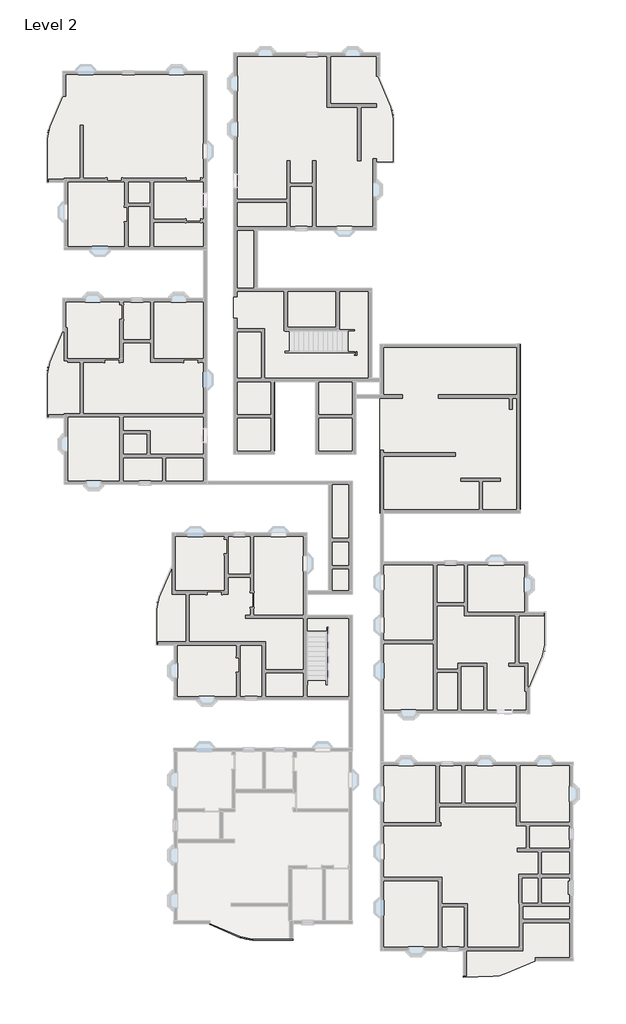
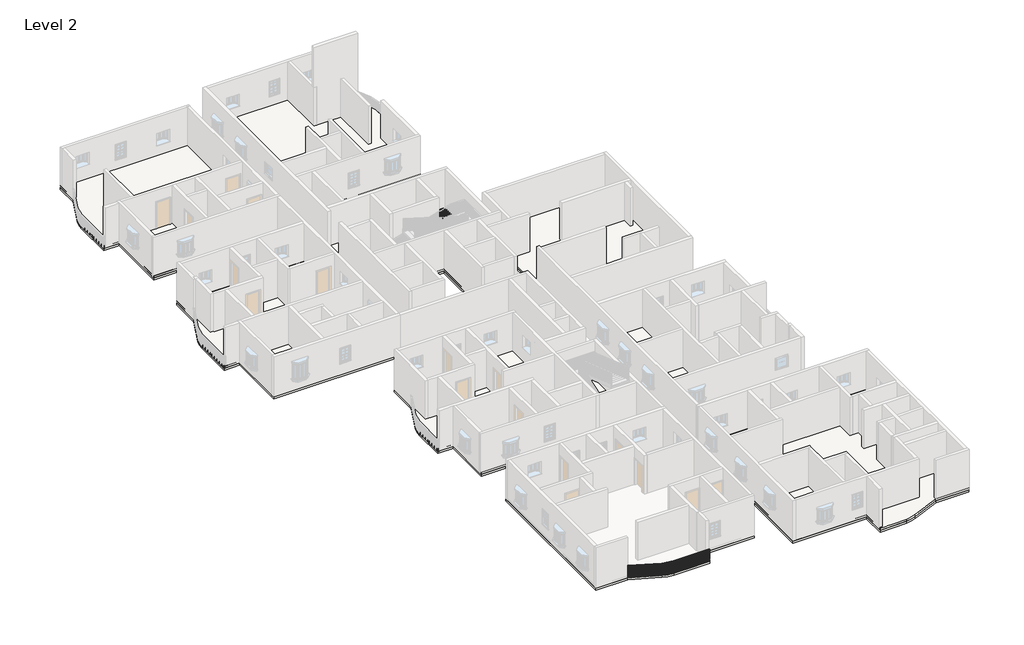
# One storey, part 5 of 14: 13 slabs, 12 roofs, 1 railing.
"""IFC4 building model written with IfcOpenShell, lengths in millimetres."""

from ifc_helpers import new_model, si_unit, point, frame, frame_2d, origin, place, context, project, spatial, polyline, circle_curve, trimmed, segment, composite_curve, outline, extrude, element, save
from ifc_brep_helpers import plane_surface, cylinder_surface, revolved_surface, advanced_brep

model = new_model("IFC4")

# Units and contexts
model_context = context("Model", 3, world=origin())
ifc_project = project(units=[si_unit("LENGTHUNIT", "METRE", prefix="MILLI")], contexts=[model_context])

# Site, building, storey
site = spatial("IfcSite", under=ifc_project)
building = spatial("IfcBuilding", under=site)
storey = spatial("IfcBuildingStorey", under=building, Name="Level 2", Elevation=3048.0)

# Railing
placement = place(None, origin())
element("IfcRailing", 1, ObjectType="Handrail - Rectangular", at=placement, inside=storey, context=model_context, shape_type="SolidModel", body=[
    advanced_brep(
    [(-10014.8722294, -25076.9923935, 3962.4), (-10014.8722294, -25076.9923935, 3911.6), (-10034.8694485, -25123.6909077, 3911.6), (-10034.8694485, -25123.6909077, 3962.4), (-8065.5370278, -25911.7359335, 3962.4), (-8065.5370278, -25911.7359335, 3911.6), (-8085.5342469, -25958.4344477, 3911.6), (-8085.5342469, -25958.4344477, 3962.4), (-7315.6413127, -26065.5416506, 3911.6), (-7315.6413127, -26065.5416506, 3962.4), (-7315.6413127, -26116.3416506, 3911.6), (-7315.6413127, -26116.3416506, 3962.4), (-4746.0891351, -26065.5416506, 3962.4), (-4746.0891351, -26116.3416506, 3962.4), (-4746.0891351, -26116.3416506, 3911.6), (-4746.0891351, -26065.5416506, 3911.6)],
    [
        (0, 1),
        (1, 2),
        (2, 3),
        (3, 0),
        (0, 4),
        (4, 5),
        (5, 1),
        (5, 6),
        (6, 2),
        (6, 7),
        (7, 3),
        (7, 4),
        (8, 5, circle_curve(frame((-7315.6413127, -24160.5416506, 3911.6), z_axis=(0.0, 0.0, -1.0), x_axis=(-0.3936460446736578, -0.9192620907623595, 0.0)), 1905.0)),
        (4, 9, circle_curve(frame((-7315.6413127, -24160.5416506, 3962.4), z_axis=(0.0, 0.0, 1.0), x_axis=(-0.3936460446736578, -0.9192620907623595, 0.0)), 1905.0)),
        (9, 8),
        (10, 6, circle_curve(frame((-7315.6413127, -24160.5416506, 3911.6), z_axis=(0.0, 0.0, -1.0), x_axis=(-0.3936460446736578, -0.9192620907623595, 0.0)), 1955.8)),
        (8, 10),
        (11, 7, circle_curve(frame((-7315.6413127, -24160.5416506, 3962.4), z_axis=(0.0, 0.0, -1.0), x_axis=(-0.3936460446736578, -0.9192620907623595, 0.0)), 1955.8)),
        (10, 11),
        (11, 9),
        (12, 13),
        (13, 14),
        (14, 15),
        (15, 12),
        (9, 12),
        (15, 8),
        (14, 10),
        (13, 11),
    ],
    [
        plane_surface(frame((-10024.8708389, -25100.3416506, 3962.4), z_axis=(-0.9192620907623597, 0.39364604467365766, 0.0), x_axis=(0.39364604467365766, 0.9192620907623597, 0.0))),
        plane_surface(frame((-10014.8722294, -25076.9923935, 3962.4), z_axis=(0.39364604467365766, 0.9192620907623597, 0.0), x_axis=(0.9192620907623597, -0.39364604467365766, 0.0))),
        plane_surface(frame((-10014.8722294, -25076.9923935, 3911.6), z_axis=(0.0, 0.0, -1.0), x_axis=(0.9192620907623597, -0.39364604467365766, 0.0))),
        plane_surface(frame((-10034.8694485, -25123.6909077, 3911.6), z_axis=(-0.39364604467365766, -0.9192620907623597, 0.0), x_axis=(0.9192620907623597, -0.39364604467365766, 0.0))),
        plane_surface(frame((-10034.8694485, -25123.6909077, 3962.4), z_axis=(0.0, 0.0, 1.0), x_axis=(0.9192620907623597, -0.39364604467365766, 0.0))),
        revolved_surface(polyline([(-8065.537027803318, -25911.735933502296, 3962.4), (-8065.537027803318, -25911.735933502296, 3911.6)]), (-7315.6413127, -24160.5416506, 3962.4), (0.0, 0.0, 1.0)),
        plane_surface(frame((-7315.6413127, -24160.5416506, 3911.6), z_axis=(0.0, 0.0, -1.0000000000000002), x_axis=(-0.3936460446736579, -0.9192620907623597, 0.0))),
        cylinder_surface(frame((-7315.6413127, -24160.5416506, 3962.4), z_axis=(0.0, 0.0, 1.0), x_axis=(-0.3936460446736578, -0.9192620907623595, 0.0)), 1955.8),
        plane_surface(frame((-7315.6413127, -24160.5416506, 3962.4), z_axis=(0.0, 0.0, 1.0000000000000002), x_axis=(-0.3936460446736579, -0.9192620907623597, 0.0))),
        plane_surface(frame((-4746.0891351, -26090.9416506, 3962.4), z_axis=(1.0, 0.0, 0.0), x_axis=(0.0, 1.0, 0.0))),
        plane_surface(frame((-7315.6413127, -26065.5416506, 3962.4), z_axis=(0.0, 1.0, 0.0), x_axis=(1.0, 0.0, 0.0))),
        plane_surface(frame((-7315.6413127, -26065.5416506, 3911.6), z_axis=(0.0, 0.0, -1.0), x_axis=(1.0, 0.0, 0.0))),
        plane_surface(frame((-7315.6413127, -26116.3416506, 3911.6), z_axis=(0.0, -1.0, 0.0), x_axis=(1.0, 0.0, 0.0))),
        plane_surface(frame((-7315.6413127, -26116.3416506, 3962.4), z_axis=(0.0, 0.0, 1.0), x_axis=(1.0, 0.0, 0.0))),
    ],
    [
        (0, [[1, 2, 3, 4]]),
        (1, [[-1, 5, 6, 7]]),
        (2, [[-2, -7, 8, 9]]),
        (3, [[-3, -9, 10, 11]]),
        (4, [[-4, -11, 12, -5]]),
        (5, [[13, -6, 14, 15]]),
        (6, [[16, -8, -13, 17]]),
        (7, [[18, -10, -16, 19]]),
        (8, [[-14, -12, -18, 20]]),
        (9, [[21, 22, 23, 24]]),
        (10, [[-15, 25, -24, 26]]),
        (11, [[-17, -26, -23, 27]]),
        (12, [[-19, -27, -22, 28]]),
        (13, [[-20, -28, -21, -25]]),
    ],
),
    extrude(outline(polyline([(-4785.1663127, -26100.4666506), (-4785.1663127, -26081.4166506), (-4766.1163127, -26081.4166506), (-4766.1163127, -26100.4666506), (-4785.1663127, -26100.4666506)])), frame((0.0, 0.0, 3048.0), z_axis=(0.0, 0.0, 1.0), x_axis=(1.0, 0.0, 0.0)), (0.0, 0.0, 1.0), 863.6),
    extrude(outline(polyline([(-4886.7663127, -26100.4666506), (-4886.7663127, -26081.4166506), (-4867.7163127, -26081.4166506), (-4867.7163127, -26100.4666506), (-4886.7663127, -26100.4666506)])), frame((0.0, 0.0, 3048.0), z_axis=(0.0, 0.0, 1.0), x_axis=(1.0, 0.0, 0.0)), (0.0, 0.0, 1.0), 863.6),
    extrude(outline(polyline([(-4988.3663127, -26100.4666506), (-4988.3663127, -26081.4166506), (-4969.3163127, -26081.4166506), (-4969.3163127, -26100.4666506), (-4988.3663127, -26100.4666506)])), frame((0.0, 0.0, 3048.0), z_axis=(0.0, 0.0, 1.0), x_axis=(1.0, 0.0, 0.0)), (0.0, 0.0, 1.0), 863.6),
    extrude(outline(polyline([(-5089.9663127, -26100.4666506), (-5089.9663127, -26081.4166506), (-5070.9163127, -26081.4166506), (-5070.9163127, -26100.4666506), (-5089.9663127, -26100.4666506)])), frame((0.0, 0.0, 3048.0), z_axis=(0.0, 0.0, 1.0), x_axis=(1.0, 0.0, 0.0)), (0.0, 0.0, 1.0), 863.6),
    extrude(outline(polyline([(-5191.5663127, -26100.4666506), (-5191.5663127, -26081.4166506), (-5172.5163127, -26081.4166506), (-5172.5163127, -26100.4666506), (-5191.5663127, -26100.4666506)])), frame((0.0, 0.0, 3048.0), z_axis=(0.0, 0.0, 1.0), x_axis=(1.0, 0.0, 0.0)), (0.0, 0.0, 1.0), 863.6),
    extrude(outline(polyline([(-5293.1663127, -26100.4666506), (-5293.1663127, -26081.4166506), (-5274.1163127, -26081.4166506), (-5274.1163127, -26100.4666506), (-5293.1663127, -26100.4666506)])), frame((0.0, 0.0, 3048.0), z_axis=(0.0, 0.0, 1.0), x_axis=(1.0, 0.0, 0.0)), (0.0, 0.0, 1.0), 863.6),
    extrude(outline(polyline([(-5394.7663127, -26100.4666506), (-5394.7663127, -26081.4166506), (-5375.7163127, -26081.4166506), (-5375.7163127, -26100.4666506), (-5394.7663127, -26100.4666506)])), frame((0.0, 0.0, 3048.0), z_axis=(0.0, 0.0, 1.0), x_axis=(1.0, 0.0, 0.0)), (0.0, 0.0, 1.0), 863.6),
    extrude(outline(polyline([(-5496.3663127, -26100.4666506), (-5496.3663127, -26081.4166506), (-5477.3163127, -26081.4166506), (-5477.3163127, -26100.4666506), (-5496.3663127, -26100.4666506)])), frame((0.0, 0.0, 3048.0), z_axis=(0.0, 0.0, 1.0), x_axis=(1.0, 0.0, 0.0)), (0.0, 0.0, 1.0), 863.6),
    extrude(outline(polyline([(-5597.9663127, -26100.4666506), (-5597.9663127, -26081.4166506), (-5578.9163127, -26081.4166506), (-5578.9163127, -26100.4666506), (-5597.9663127, -26100.4666506)])), frame((0.0, 0.0, 3048.0), z_axis=(0.0, 0.0, 1.0), x_axis=(1.0, 0.0, 0.0)), (0.0, 0.0, 1.0), 863.6),
    extrude(outline(polyline([(-5699.5663127, -26100.4666506), (-5699.5663127, -26081.4166506), (-5680.5163127, -26081.4166506), (-5680.5163127, -26100.4666506), (-5699.5663127, -26100.4666506)])), frame((0.0, 0.0, 3048.0), z_axis=(0.0, 0.0, 1.0), x_axis=(1.0, 0.0, 0.0)), (0.0, 0.0, 1.0), 863.6),
    extrude(outline(polyline([(-5801.1663127, -26100.4666506), (-5801.1663127, -26081.4166506), (-5782.1163127, -26081.4166506), (-5782.1163127, -26100.4666506), (-5801.1663127, -26100.4666506)])), frame((0.0, 0.0, 3048.0), z_axis=(0.0, 0.0, 1.0), x_axis=(1.0, 0.0, 0.0)), (0.0, 0.0, 1.0), 863.6),
    extrude(outline(polyline([(-5902.7663127, -26100.4666506), (-5902.7663127, -26081.4166506), (-5883.7163127, -26081.4166506), (-5883.7163127, -26100.4666506), (-5902.7663127, -26100.4666506)])), frame((0.0, 0.0, 3048.0), z_axis=(0.0, 0.0, 1.0), x_axis=(1.0, 0.0, 0.0)), (0.0, 0.0, 1.0), 863.6),
    extrude(outline(polyline([(-6004.3663127, -26100.4666506), (-6004.3663127, -26081.4166506), (-5985.3163127, -26081.4166506), (-5985.3163127, -26100.4666506), (-6004.3663127, -26100.4666506)])), frame((0.0, 0.0, 3048.0), z_axis=(0.0, 0.0, 1.0), x_axis=(1.0, 0.0, 0.0)), (0.0, 0.0, 1.0), 863.6),
    extrude(outline(polyline([(-6105.9663127, -26100.4666506), (-6105.9663127, -26081.4166506), (-6086.9163127, -26081.4166506), (-6086.9163127, -26100.4666506), (-6105.9663127, -26100.4666506)])), frame((0.0, 0.0, 3048.0), z_axis=(0.0, 0.0, 1.0), x_axis=(1.0, 0.0, 0.0)), (0.0, 0.0, 1.0), 863.6),
    extrude(outline(polyline([(-6207.5663127, -26100.4666506), (-6207.5663127, -26081.4166506), (-6188.5163127, -26081.4166506), (-6188.5163127, -26100.4666506), (-6207.5663127, -26100.4666506)])), frame((0.0, 0.0, 3048.0), z_axis=(0.0, 0.0, 1.0), x_axis=(1.0, 0.0, 0.0)), (0.0, 0.0, 1.0), 863.6),
    extrude(outline(polyline([(-6309.1663127, -26100.4666506), (-6309.1663127, -26081.4166506), (-6290.1163127, -26081.4166506), (-6290.1163127, -26100.4666506), (-6309.1663127, -26100.4666506)])), frame((0.0, 0.0, 3048.0), z_axis=(0.0, 0.0, 1.0), x_axis=(1.0, 0.0, 0.0)), (0.0, 0.0, 1.0), 863.6),
    extrude(outline(polyline([(-6410.7663127, -26100.4666506), (-6410.7663127, -26081.4166506), (-6391.7163127, -26081.4166506), (-6391.7163127, -26100.4666506), (-6410.7663127, -26100.4666506)])), frame((0.0, 0.0, 3048.0), z_axis=(0.0, 0.0, 1.0), x_axis=(1.0, 0.0, 0.0)), (0.0, 0.0, 1.0), 863.6),
    extrude(outline(polyline([(-6512.3663127, -26100.4666506), (-6512.3663127, -26081.4166506), (-6493.3163127, -26081.4166506), (-6493.3163127, -26100.4666506), (-6512.3663127, -26100.4666506)])), frame((0.0, 0.0, 3048.0), z_axis=(0.0, 0.0, 1.0), x_axis=(1.0, 0.0, 0.0)), (0.0, 0.0, 1.0), 863.6),
    extrude(outline(polyline([(-6613.9663127, -26100.4666506), (-6613.9663127, -26081.4166506), (-6594.9163127, -26081.4166506), (-6594.9163127, -26100.4666506), (-6613.9663127, -26100.4666506)])), frame((0.0, 0.0, 3048.0), z_axis=(0.0, 0.0, 1.0), x_axis=(1.0, 0.0, 0.0)), (0.0, 0.0, 1.0), 863.6),
    extrude(outline(polyline([(-6715.5663127, -26100.4666506), (-6715.5663127, -26081.4166506), (-6696.5163127, -26081.4166506), (-6696.5163127, -26100.4666506), (-6715.5663127, -26100.4666506)])), frame((0.0, 0.0, 3048.0), z_axis=(0.0, 0.0, 1.0), x_axis=(1.0, 0.0, 0.0)), (0.0, 0.0, 1.0), 863.6),
    extrude(outline(polyline([(-6817.1663127, -26100.4666506), (-6817.1663127, -26081.4166506), (-6798.1163127, -26081.4166506), (-6798.1163127, -26100.4666506), (-6817.1663127, -26100.4666506)])), frame((0.0, 0.0, 3048.0), z_axis=(0.0, 0.0, 1.0), x_axis=(1.0, 0.0, 0.0)), (0.0, 0.0, 1.0), 863.6),
    extrude(outline(polyline([(-6918.7663127, -26100.4666506), (-6918.7663127, -26081.4166506), (-6899.7163127, -26081.4166506), (-6899.7163127, -26100.4666506), (-6918.7663127, -26100.4666506)])), frame((0.0, 0.0, 3048.0), z_axis=(0.0, 0.0, 1.0), x_axis=(1.0, 0.0, 0.0)), (0.0, 0.0, 1.0), 863.6),
    extrude(outline(polyline([(-7020.3663127, -26100.4666506), (-7020.3663127, -26081.4166506), (-7001.3163127, -26081.4166506), (-7001.3163127, -26100.4666506), (-7020.3663127, -26100.4666506)])), frame((0.0, 0.0, 3048.0), z_axis=(0.0, 0.0, 1.0), x_axis=(1.0, 0.0, 0.0)), (0.0, 0.0, 1.0), 863.6),
    extrude(outline(polyline([(-7121.9663127, -26100.4666506), (-7121.9663127, -26081.4166506), (-7102.9163127, -26081.4166506), (-7102.9163127, -26100.4666506), (-7121.9663127, -26100.4666506)])), frame((0.0, 0.0, 3048.0), z_axis=(0.0, 0.0, 1.0), x_axis=(1.0, 0.0, 0.0)), (0.0, 0.0, 1.0), 863.6),
    extrude(outline(polyline([(-7223.5663127, -26100.4666506), (-7223.5663127, -26081.4166506), (-7204.5163127, -26081.4166506), (-7204.5163127, -26100.4666506), (-7223.5663127, -26100.4666506)])), frame((0.0, 0.0, 3048.0), z_axis=(0.0, 0.0, 1.0), x_axis=(1.0, 0.0, 0.0)), (0.0, 0.0, 1.0), 863.6),
    extrude(outline(polyline([(-7395.3185803, -26098.8530973), (-7394.6296262, -26079.8155596), (-7375.5920885, -26080.5045137), (-7376.2810426, -26099.5420514), (-7395.3185803, -26098.8530973)])), frame((0.0, 0.0, 3048.0), z_axis=(0.0, 0.0, 1.0), x_axis=(1.0, 0.0, 0.0)), (0.0, 0.0, 1.0), 863.6),
    extrude(outline(polyline([(-7497.177549, -26091.9774704), (-7495.4880357, -26073.0025384), (-7476.5131037, -26074.6920517), (-7478.2026169, -26093.6669837), (-7497.177549, -26091.9774704)])), frame((0.0, 0.0, 3048.0), z_axis=(0.0, 0.0, 1.0), x_axis=(1.0, 0.0, 0.0)), (0.0, 0.0, 1.0), 863.6),
    extrude(outline(polyline([(-7598.5337632, -26079.7528408), (-7595.8483698, -26060.8930645), (-7576.9885935, -26063.5784579), (-7579.6739869, -26082.4382342), (-7598.5337632, -26079.7528408)])), frame((0.0, 0.0, 3048.0), z_axis=(0.0, 0.0, 1.0), x_axis=(1.0, 0.0, 0.0)), (0.0, 0.0, 1.0), 863.6),
    extrude(outline(polyline([(-7699.1065227, -26062.2130639), (-7695.4326862, -26043.5206744), (-7676.7402967, -26047.1945108), (-7680.4141332, -26065.8869003), (-7699.1065227, -26062.2130639)])), frame((0.0, 0.0, 3048.0), z_axis=(0.0, 0.0, 1.0), x_axis=(1.0, 0.0, 0.0)), (0.0, 0.0, 1.0), 863.6),
    extrude(outline(polyline([(-7798.6172969, -26039.4067149), (-7793.9651918, -26020.9334797), (-7775.4919566, -26025.5855848), (-7780.1440617, -26044.05882), (-7798.6172969, -26039.4067149)])), frame((0.0, 0.0, 3048.0), z_axis=(0.0, 0.0, 1.0), x_axis=(1.0, 0.0, 0.0)), (0.0, 0.0, 1.0), 863.6),
    extrude(outline(polyline([(-7896.7904963, -26011.396955), (-7891.1730064, -25993.1940347), (-7872.9700861, -25998.8115246), (-7878.587576, -26017.0144449), (-7896.7904963, -26011.396955)])), frame((0.0, 0.0, 3048.0), z_axis=(0.0, 0.0, 1.0), x_axis=(1.0, 0.0, 0.0)), (0.0, 0.0, 1.0), 863.6),
    extrude(outline(polyline([(-7993.3542357, -25978.2613554), (-7986.7869183, -25960.379162), (-7968.9047249, -25966.9464794), (-7975.4720423, -25984.8286729), (-7993.3542357, -25978.2613554)])), frame((0.0, 0.0, 3048.0), z_axis=(0.0, 0.0, 1.0), x_axis=(1.0, 0.0, 0.0)), (0.0, 0.0, 1.0), 863.6),
    extrude(outline(polyline([(-8169.4357205, -25905.2369062), (-8161.9367633, -25887.7249634), (-8144.4248205, -25895.2239205), (-8151.9237777, -25912.7358634), (-8169.4357205, -25905.2369062)])), frame((0.0, 0.0, 3048.0), z_axis=(0.0, 0.0, 1.0), x_axis=(1.0, 0.0, 0.0)), (0.0, 0.0, 1.0), 863.6),
    extrude(outline(polyline([(-8262.8327489, -25865.2424681), (-8255.3337918, -25847.7305252), (-8237.8218489, -25855.2294824), (-8245.3208061, -25872.7414252), (-8262.8327489, -25865.2424681)])), frame((0.0, 0.0, 3048.0), z_axis=(0.0, 0.0, 1.0), x_axis=(1.0, 0.0, 0.0)), (0.0, 0.0, 1.0), 863.6),
    extrude(outline(polyline([(-8356.2297773, -25825.2480299), (-8348.7308202, -25807.7360871), (-8331.2188774, -25815.2350443), (-8338.7178345, -25832.7469871), (-8356.2297773, -25825.2480299)])), frame((0.0, 0.0, 3048.0), z_axis=(0.0, 0.0, 1.0), x_axis=(1.0, 0.0, 0.0)), (0.0, 0.0, 1.0), 863.6),
    extrude(outline(polyline([(-8449.6268058, -25785.2535918), (-8442.1278486, -25767.741649), (-8424.6159058, -25775.2406061), (-8432.1148629, -25792.752549), (-8449.6268058, -25785.2535918)])), frame((0.0, 0.0, 3048.0), z_axis=(0.0, 0.0, 1.0), x_axis=(1.0, 0.0, 0.0)), (0.0, 0.0, 1.0), 863.6),
    extrude(outline(polyline([(-8543.0238342, -25745.2591537), (-8535.524877, -25727.7472108), (-8518.0129342, -25735.246168), (-8525.5118914, -25752.7581108), (-8543.0238342, -25745.2591537)])), frame((0.0, 0.0, 3048.0), z_axis=(0.0, 0.0, 1.0), x_axis=(1.0, 0.0, 0.0)), (0.0, 0.0, 1.0), 863.6),
    extrude(outline(polyline([(-8636.4208626, -25705.2647155), (-8628.9219055, -25687.7527727), (-8611.4099626, -25695.2517298), (-8618.9089198, -25712.7636727), (-8636.4208626, -25705.2647155)])), frame((0.0, 0.0, 3048.0), z_axis=(0.0, 0.0, 1.0), x_axis=(1.0, 0.0, 0.0)), (0.0, 0.0, 1.0), 863.6),
    extrude(outline(polyline([(-8729.817891, -25665.2702774), (-8722.3189339, -25647.7583346), (-8704.806991, -25655.2572917), (-8712.3059482, -25672.7692345), (-8729.817891, -25665.2702774)])), frame((0.0, 0.0, 3048.0), z_axis=(0.0, 0.0, 1.0), x_axis=(1.0, 0.0, 0.0)), (0.0, 0.0, 1.0), 863.6),
    extrude(outline(polyline([(-8823.2149194, -25625.2758392), (-8815.7159623, -25607.7638964), (-8798.2040195, -25615.2628536), (-8805.7029766, -25632.7747964), (-8823.2149194, -25625.2758392)])), frame((0.0, 0.0, 3048.0), z_axis=(0.0, 0.0, 1.0), x_axis=(1.0, 0.0, 0.0)), (0.0, 0.0, 1.0), 863.6),
    extrude(outline(polyline([(-8916.6119479, -25585.2814011), (-8909.1129907, -25567.7694583), (-8891.6010479, -25575.2684154), (-8899.100005, -25592.7803583), (-8916.6119479, -25585.2814011)])), frame((0.0, 0.0, 3048.0), z_axis=(0.0, 0.0, 1.0), x_axis=(1.0, 0.0, 0.0)), (0.0, 0.0, 1.0), 863.6),
    extrude(outline(polyline([(-9010.0089763, -25545.286963), (-9002.5100191, -25527.7750201), (-8984.9980763, -25535.2739773), (-8992.4970335, -25552.7859201), (-9010.0089763, -25545.286963)])), frame((0.0, 0.0, 3048.0), z_axis=(0.0, 0.0, 1.0), x_axis=(1.0, 0.0, 0.0)), (0.0, 0.0, 1.0), 863.6),
    extrude(outline(polyline([(-9103.4060047, -25505.2925248), (-9095.9070476, -25487.780582), (-9078.3951047, -25495.2795391), (-9085.8940619, -25512.791482), (-9103.4060047, -25505.2925248)])), frame((0.0, 0.0, 3048.0), z_axis=(0.0, 0.0, 1.0), x_axis=(1.0, 0.0, 0.0)), (0.0, 0.0, 1.0), 863.6),
    extrude(outline(polyline([(-9196.8030331, -25465.2980867), (-9189.304076, -25447.7861439), (-9171.7921332, -25455.285101), (-9179.2910903, -25472.7970438), (-9196.8030331, -25465.2980867)])), frame((0.0, 0.0, 3048.0), z_axis=(0.0, 0.0, 1.0), x_axis=(1.0, 0.0, 0.0)), (0.0, 0.0, 1.0), 863.6),
    extrude(outline(polyline([(-9290.2000616, -25425.3036485), (-9282.7011044, -25407.7917057), (-9265.1891616, -25415.2906629), (-9272.6881187, -25432.8026057), (-9290.2000616, -25425.3036485)])), frame((0.0, 0.0, 3048.0), z_axis=(0.0, 0.0, 1.0), x_axis=(1.0, 0.0, 0.0)), (0.0, 0.0, 1.0), 863.6),
    extrude(outline(polyline([(-9383.59709, -25385.3092104), (-9376.0981328, -25367.7972676), (-9358.58619, -25375.2962247), (-9366.0851471, -25392.8081676), (-9383.59709, -25385.3092104)])), frame((0.0, 0.0, 3048.0), z_axis=(0.0, 0.0, 1.0), x_axis=(1.0, 0.0, 0.0)), (0.0, 0.0, 1.0), 863.6),
    extrude(outline(polyline([(-9476.9941184, -25345.3147723), (-9469.4951612, -25327.8028294), (-9451.9832184, -25335.3017866), (-9459.4821756, -25352.8137294), (-9476.9941184, -25345.3147723)])), frame((0.0, 0.0, 3048.0), z_axis=(0.0, 0.0, 1.0), x_axis=(1.0, 0.0, 0.0)), (0.0, 0.0, 1.0), 863.6),
    extrude(outline(polyline([(-9570.3911468, -25305.3203341), (-9562.8921897, -25287.8083913), (-9545.3802468, -25295.3073485), (-9552.879204, -25312.8192913), (-9570.3911468, -25305.3203341)])), frame((0.0, 0.0, 3048.0), z_axis=(0.0, 0.0, 1.0), x_axis=(1.0, 0.0, 0.0)), (0.0, 0.0, 1.0), 863.6),
    extrude(outline(polyline([(-9663.7881752, -25265.325896), (-9656.2892181, -25247.8139532), (-9638.7772753, -25255.3129103), (-9646.2762324, -25272.8248531), (-9663.7881752, -25265.325896)])), frame((0.0, 0.0, 3048.0), z_axis=(0.0, 0.0, 1.0), x_axis=(1.0, 0.0, 0.0)), (0.0, 0.0, 1.0), 863.6),
    extrude(outline(polyline([(-9757.1852037, -25225.3314579), (-9749.6862465, -25207.819515), (-9732.1743037, -25215.3184722), (-9739.6732608, -25232.830415), (-9757.1852037, -25225.3314579)])), frame((0.0, 0.0, 3048.0), z_axis=(0.0, 0.0, 1.0), x_axis=(1.0, 0.0, 0.0)), (0.0, 0.0, 1.0), 863.6),
    extrude(outline(polyline([(-9850.5822321, -25185.3370197), (-9843.0832749, -25167.8250769), (-9825.5713321, -25175.324034), (-9833.0702893, -25192.8359769), (-9850.5822321, -25185.3370197)])), frame((0.0, 0.0, 3048.0), z_axis=(0.0, 0.0, 1.0), x_axis=(1.0, 0.0, 0.0)), (0.0, 0.0, 1.0), 863.6),
    extrude(outline(polyline([(-9943.9792605, -25145.3425816), (-9936.4803034, -25127.8306387), (-9918.9683605, -25135.3295959), (-9926.4673177, -25152.8415387), (-9943.9792605, -25145.3425816)])), frame((0.0, 0.0, 3048.0), z_axis=(0.0, 0.0, 1.0), x_axis=(1.0, 0.0, 0.0)), (0.0, 0.0, 1.0), 863.6),
    extrude(outline(polyline([(-7325.1663127, -26100.4666506), (-7325.1663127, -26081.4166506), (-7306.1163127, -26081.4166506), (-7306.1163127, -26100.4666506), (-7325.1663127, -26100.4666506)])), frame((0.0, 0.0, 3048.0), z_axis=(0.0, 0.0, 1.0), x_axis=(1.0, 0.0, 0.0)), (0.0, 0.0, 1.0), 863.6),
    extrude(outline(polyline([(-8088.0410874, -25940.0916834), (-8080.5421302, -25922.5797406), (-8063.0301874, -25930.0786978), (-8070.5291445, -25947.5906406), (-8088.0410874, -25940.0916834)])), frame((0.0, 0.0, 3048.0), z_axis=(0.0, 0.0, 1.0), x_axis=(1.0, 0.0, 0.0)), (0.0, 0.0, 1.0), 863.6),
    extrude(outline(polyline([(-4765.1391351, -26100.4666506), (-4765.1391351, -26081.4166506), (-4746.0891351, -26081.4166506), (-4746.0891351, -26100.4666506), (-4765.1391351, -26100.4666506)])), frame((0.0, 0.0, 3048.0), z_axis=(0.0, 0.0, 1.0), x_axis=(1.0, 0.0, 0.0)), (0.0, 0.0, 1.0), 863.6),
    extrude(outline(polyline([(-10028.6203175, -25109.097622), (-10021.1213604, -25091.5856792), (-10003.6094175, -25099.0846363), (-10011.1083747, -25116.5965792), (-10028.6203175, -25109.097622)])), frame((0.0, 0.0, 3048.0), z_axis=(0.0, 0.0, 1.0), x_axis=(1.0, 0.0, 0.0)), (0.0, 0.0, 1.0), 863.6),
])

# Roofs
element("IfcRoof", 2, ObjectType="Generic - 12\"", at=placement, inside=storey, context=model_context, shape_type="SweptSolid", body=[
    extrude(outline(composite_curve([segment(polyline([(6070.4380523, -26783.9042694), (812.6380523, -26783.9042694), (812.6380523, -14845.9042694), (13017.3380523, -14845.9042694), (13017.3380523, -27431.6042694), (10660.5280667, -27431.6042694), (8711.1928652, -28266.3478094)]), True, "CONTINUOUS"), segment(trimmed(circle_curve(frame_2d((7951.2985405, -26491.8042694)), 1930.4), [point((8711.1928652, -28266.3478094))], [point((7953.0959373, -28422.2034326))], False, "CARTESIAN"), True, "CONTINUOUS"), segment(polyline([(7953.0959373, -28422.2034326), (6070.4380523, -28487.9472947), (6070.4380523, -26783.9042694)]), True, "CONTINUOUS")], self_intersect=False)), frame((0.0, 0.0, 3048.0), z_axis=(0.0, 0.0, 1.0), x_axis=(1.0, 0.0, 0.0)), (0.0, 0.0, 1.0), 152.4),
])
element("IfcRoof", 3, ObjectType="Generic - 12\"", at=placement, inside=storey, context=model_context, shape_type="SweptSolid", body=[
    extrude(outline(composite_curve([segment(polyline([(10274.1380523, -11759.8042694), (803.8108649, -11759.8042694), (803.8108649, -2133.2042694), (10159.8380523, -2133.2042694), (10159.8380523, -5352.6542694), (11264.7380523, -5352.6542694), (11264.7380523, -7397.5810633)]), True, "CONTINUOUS"), segment(trimmed(circle_curve(frame_2d((9334.3380523, -7397.5810633)), 1930.4), [point((11264.7380523, -7397.5810633))], [point((11108.8815923, -8157.475388))], False, "CARTESIAN"), True, "CONTINUOUS"), segment(polyline([(11108.8815923, -8157.475388), (10274.1380523, -10106.8105895), (10274.1380523, -11759.8042694)]), True, "CONTINUOUS")], self_intersect=False)), frame((0.0, 0.0, 3048.0), z_axis=(0.0, 0.0, 1.0), x_axis=(1.0, 0.0, 0.0)), (0.0, 0.0, 1.0), 152.4),
])
element("IfcRoof", 4, ObjectType="Generic - 12\"", at=placement, inside=storey, context=model_context, shape_type="SweptSolid", body=[
    extrude(outline(composite_curve([segment(polyline([(-13395.387215, -7421.9416506), (-13395.387215, -5140.4900045)]), True, "CONTINUOUS"), segment(trimmed(circle_curve(frame_2d((-11464.987215, -5140.4900045)), 1930.4), [point((-13395.387215, -5140.4900045))], [point((-13239.530755, -4380.5956799))], False, "CARTESIAN"), True, "CONTINUOUS"), segment(polyline([(-13239.530755, -4380.5956799), (-12404.787215, -2431.2604783), (-12404.787215, -322.6416506), (-3857.687215, -322.6416506), (-3857.687215, -5523.2916506), (-974.1891351, -5523.2916506), (-974.1891351, -10889.0416506), (-12290.487215, -10889.0416506), (-12290.487215, -7421.9416506), (-13395.387215, -7421.9416506)]), True, "CONTINUOUS")], self_intersect=False)), frame((0.0, 0.0, 3048.0), z_axis=(0.0, 0.0, 1.0), x_axis=(1.0, 0.0, 0.0)), (0.0, 0.0, 1.0), 152.4),
])
element("IfcRoof", 5, ObjectType="Generic - 12\"", at=placement, inside=storey, context=model_context, shape_type="SweptSolid", body=[
    extrude(outline(polyline([(-2472.7891351, 2953.9583494), (-961.4891351, 2953.9583494), (-961.4891351, -4202.4916506), (-2472.7891351, -4202.4916506), (-2472.7891351, 2953.9583494)])), frame((0.0, 0.0, 3048.0), z_axis=(0.0, 0.0, 1.0), x_axis=(1.0, 0.0, 0.0)), (0.0, 0.0, 1.0), 152.4),
])
element("IfcRoof", 6, ObjectType="Generic - 12\"", at=placement, inside=storey, context=model_context, shape_type="SweptSolid", body=[
    extrude(outline(composite_curve([segment(polyline([(-10194.3891351, 2750.7583494), (-19236.7891351, 2750.7583494), (-19236.7891351, 6979.8583494), (-20341.6891351, 6979.8583494), (-20341.6891351, 9746.7948172)]), True, "CONTINUOUS"), segment(trimmed(circle_curve(frame_2d((-18411.2891351, 9746.7948172)), 1930.4), [point((-20341.6891351, 9746.7948172))], [point((-20185.8326751, 10506.6891419))], False, "CARTESIAN"), True, "CONTINUOUS"), segment(polyline([(-20185.8326751, 10506.6891419), (-19351.0891351, 12456.0243434), (-19351.0891351, 14536.3583494), (-10194.3891351, 14536.3583494), (-10194.3891351, 2750.7583494)]), True, "CONTINUOUS")], self_intersect=False)), frame((0.0, 0.0, 3048.0), z_axis=(0.0, 0.0, 1.0), x_axis=(1.0, 0.0, 0.0)), (0.0, 0.0, 1.0), 152.4),
])
element("IfcRoof", 7, ObjectType="Generic - 12\"", at=placement, inside=storey, context=model_context, shape_type="SweptSolid", body=[
    extrude(outline(composite_curve([segment(polyline([(-10194.3891351, 17609.7583494), (-19236.7891351, 17609.7583494), (-19236.7891351, 21889.6583494), (-20341.6891351, 21889.6583494), (-20341.6891351, 24656.5948172)]), True, "CONTINUOUS"), segment(trimmed(circle_curve(frame_2d((-18411.2891351, 24656.5948172)), 1930.4), [point((-20341.6891351, 24656.5948172))], [point((-20185.8326751, 25416.4891419))], False, "CARTESIAN"), True, "CONTINUOUS"), segment(polyline([(-20185.8326751, 25416.4891419), (-19351.0891351, 27365.8243434), (-19351.0891351, 28950.8583494), (-10194.3891351, 28950.8583494), (-10194.3891351, 17609.7583494)]), True, "CONTINUOUS")], self_intersect=False)), frame((0.0, 0.0, 3048.0), z_axis=(0.0, 0.0, 1.0), x_axis=(1.0, 0.0, 0.0)), (0.0, 0.0, 1.0), 152.4),
])
element("IfcRoof", 8, ObjectType="Generic - 12\"", at=placement, inside=storey, context=model_context, shape_type="SweptSolid", body=[
    extrude(outline(composite_curve([segment(polyline([(-8492.5891351, 18875.1215905), (-8492.5891351, 30101.9215905), (664.1108649, 30101.9215905), (664.1108649, 28631.1875845), (1498.8544049, 26681.8523829)]), True, "CONTINUOUS"), segment(trimmed(circle_curve(frame_2d((-275.6891351, 25921.9580583)), 1930.4), [point((1498.8544049, 26681.8523829))], [point((1654.7108649, 25921.9580583))], False, "CARTESIAN"), True, "CONTINUOUS"), segment(polyline([(1654.7108649, 25921.9580583), (1654.7108649, 23155.0215905), (549.8108649, 23155.0215905), (549.8108649, 18875.1215905), (-8492.5891351, 18875.1215905)]), True, "CONTINUOUS")], self_intersect=False)), frame((0.0, 0.0, 3048.0), z_axis=(0.0, 0.0, 1.0), x_axis=(1.0, 0.0, 0.0)), (0.0, 0.0, 1.0), 152.4),
])
element("IfcRoof", 9, ObjectType="Generic - 12\"", at=placement, inside=storey, context=model_context, shape_type="SweptSolid", body=[
    extrude(outline(polyline([(-8492.5891351, 9478.4949943), (-5914.4891351, 9478.4949943), (-5914.4891351, 4665.1949943), (-8492.5891351, 4665.1949943), (-8492.5891351, 9478.4949943)])), frame((0.0, 0.0, 3048.0), z_axis=(0.0, 0.0, 1.0), x_axis=(1.0, 0.0, 0.0)), (0.0, 0.0, 1.0), 152.4),
])
element("IfcRoof", 10, ObjectType="Generic - 12\"", at=placement, inside=storey, context=model_context, shape_type="SweptSolid", body=[
    extrude(outline(polyline([(-3310.9891351, 9478.4949943), (-745.5891351, 9478.4949943), (-745.5891351, 4652.4949943), (-3310.9891351, 4652.4949943), (-3310.9891351, 9478.4949943)])), frame((0.0, 0.0, 3048.0), z_axis=(0.0, 0.0, 1.0), x_axis=(1.0, 0.0, 0.0)), (0.0, 0.0, 1.0), 152.4),
])
element("IfcRoof", 11, ObjectType="Generic - 12\"", at=placement, inside=storey, context=model_context, shape_type="SweptSolid", body=[
    extrude(outline(polyline([(-8492.5891351, 19078.3215905), (-6993.9891351, 19078.3215905), (-6993.9891351, 14988.9215905), (-8492.5891351, 14988.9215905), (-8492.5891351, 19078.3215905)])), frame((0.0, 0.0, 3048.0), z_axis=(0.0, 0.0, 1.0), x_axis=(1.0, 0.0, 0.0)), (0.0, 0.0, 1.0), 152.4),
])
element("IfcRoof", 12, ObjectType="Generic - 12\"", at=placement, inside=storey, context=model_context, shape_type="SweptSolid", body=[
    extrude(outline(polyline([(-8492.5891351, 15192.1215905), (257.7108649, 15192.1215905), (257.7108649, 9275.2949943), (-8492.5891351, 9275.2949943), (-8492.5891351, 15192.1215905)])), frame((0.0, 0.0, 3048.0), z_axis=(0.0, 0.0, 1.0), x_axis=(1.0, 0.0, 0.0)), (0.0, 0.0, 1.0), 152.4),
])
element("IfcRoof", 13, ObjectType="Generic - 12\"", at=placement, inside=storey, context=model_context, shape_type="SweptSolid", body=[
    extrude(outline(polyline([(793.5880523, 11646.2957306), (9677.2380523, 11646.2957306), (9677.2380523, 940.1957306), (793.5880523, 940.1957306), (793.5880523, 11646.2957306)])), frame((0.0, 0.0, 3048.0), z_axis=(0.0, 0.0, 1.0), x_axis=(1.0, 0.0, 0.0)), (0.0, 0.0, 1.0), 152.4),
])

# Slabs
element("IfcSlab", 14, ObjectType="Generic - 12\"", at=placement, inside=storey, context=model_context, shape_type="SweptSolid", body=[
    extrude(outline(composite_curve([segment(polyline([(-20341.6891351, 21889.6583494), (-20341.6891351, 24656.5948172)]), True, "CONTINUOUS"), segment(trimmed(circle_curve(frame_2d((-18411.2891351, 24656.5948172)), 1930.4), [point((-20341.6891351, 24656.5948172))], [point((-20185.8326751, 25416.4891419))], False, "CARTESIAN"), True, "CONTINUOUS"), segment(polyline([(-20185.8326751, 25416.4891419), (-19351.0891351, 27365.8243434), (-19351.0891351, 28950.8583494), (-10194.3891351, 28950.8583494), (-10194.3891351, 17609.7583494), (-19236.7891351, 17609.7583494), (-19236.7891351, 21889.6583494), (-20341.6891351, 21889.6583494)]), True, "CONTINUOUS")], self_intersect=False)), frame((0.0, 0.0, 2895.6), z_axis=(0.0, 0.0, 1.0), x_axis=(1.0, 0.0, 0.0)), (0.0, 0.0, 1.0), 152.4),
])
element("IfcSlab", 15, ObjectType="Generic - 12\"", at=placement, inside=storey, context=model_context, shape_type="SweptSolid", body=[
    extrude(outline(composite_curve([segment(polyline([(-10024.8708389, -25100.3416506), (-12290.487215, -25100.3416506), (-12290.487215, -13962.4416506), (-986.8891351, -13962.4416506), (-986.8891351, -25100.3416506), (-4746.0891351, -25100.3416506), (-4746.0891351, -26090.9416506), (-7315.6413127, -26090.9416506)]), True, "CONTINUOUS"), segment(trimmed(circle_curve(frame_2d((-7315.6413127, -24160.5416506)), 1930.4), [point((-7315.6413127, -26090.9416506))], [point((-8075.5356374, -25935.0851906))], False, "CARTESIAN"), True, "CONTINUOUS"), segment(polyline([(-8075.5356374, -25935.0851906), (-10024.8708389, -25100.3416506)]), True, "CONTINUOUS")], self_intersect=False)), frame((0.0, 0.0, 2895.6), z_axis=(0.0, 0.0, 1.0), x_axis=(1.0, 0.0, 0.0)), (0.0, 0.0, 1.0), 152.4),
])
element("IfcSlab", 16, ObjectType="Generic - 12\"", at=placement, inside=storey, context=model_context, shape_type="SweptSolid", body=[
    extrude(outline(composite_curve([segment(polyline([(13017.3380523, -27431.6042694), (10660.5280667, -27431.6042694), (8711.1928652, -28266.3478094)]), True, "CONTINUOUS"), segment(trimmed(circle_curve(frame_2d((7951.2985405, -26491.8042694)), 1930.4), [point((8711.1928652, -28266.3478094))], [point((7953.0959373, -28422.2034326))], False, "CARTESIAN"), True, "CONTINUOUS"), segment(polyline([(7953.0959373, -28422.2034326), (6070.4380523, -28487.9472947), (6070.4380523, -26783.9042694), (812.6380523, -26783.9042694), (812.6380523, -14845.9042694), (13017.3380523, -14845.9042694), (13017.3380523, -27431.6042694)]), True, "CONTINUOUS")], self_intersect=False)), frame((0.0, 0.0, 2895.6), z_axis=(0.0, 0.0, 1.0), x_axis=(1.0, 0.0, 0.0)), (0.0, 0.0, 1.0), 152.4),
])
element("IfcSlab", 17, ObjectType="Generic - 12\"", at=placement, inside=storey, context=model_context, shape_type="SweptSolid", body=[
    extrude(outline(composite_curve([segment(polyline([(10274.1380523, -11759.8042694), (803.8108649, -11759.8042694), (803.8108649, -2133.2042694), (10159.8380523, -2133.2042694), (10159.8380523, -5352.6542694), (11264.7380523, -5352.6542694), (11264.7380523, -7397.5810633)]), True, "CONTINUOUS"), segment(trimmed(circle_curve(frame_2d((9334.3380523, -7397.5810633)), 1930.4), [point((11264.7380523, -7397.5810633))], [point((11108.8815923, -8157.475388))], False, "CARTESIAN"), True, "CONTINUOUS"), segment(polyline([(11108.8815923, -8157.475388), (10274.1380523, -10106.8105895), (10274.1380523, -11759.8042694)]), True, "CONTINUOUS")], self_intersect=False)), frame((0.0, 0.0, 2895.6), z_axis=(0.0, 0.0, 1.0), x_axis=(1.0, 0.0, 0.0)), (0.0, 0.0, 1.0), 152.4),
])
element("IfcSlab", 18, ObjectType="Generic - 12\"", at=placement, inside=storey, context=model_context, shape_type="SweptSolid", body=[
    extrude(outline(composite_curve([segment(polyline([(-974.1891351, -10889.0416506), (-12290.487215, -10889.0416506), (-12290.487215, -7421.9416506), (-13395.387215, -7421.9416506), (-13395.387215, -5140.4900045)]), True, "CONTINUOUS"), segment(trimmed(circle_curve(frame_2d((-11464.987215, -5140.4900045)), 1930.4), [point((-13395.387215, -5140.4900045))], [point((-13239.530755, -4380.5956799))], False, "CARTESIAN"), True, "CONTINUOUS"), segment(polyline([(-13239.530755, -4380.5956799), (-12404.787215, -2431.2604783), (-12404.787215, -322.6416506), (-3857.687215, -322.6416506), (-3857.687215, -5523.2916506), (-974.1891351, -5523.2916506), (-974.1891351, -10889.0416506)]), True, "CONTINUOUS")], self_intersect=False)), frame((0.0, 0.0, 2895.6), z_axis=(0.0, 0.0, 1.0), x_axis=(1.0, 0.0, 0.0)), (0.0, 0.0, 1.0), 152.4),
])
element("IfcSlab", 19, ObjectType="Generic - 12\"", at=placement, inside=storey, context=model_context, shape_type="SweptSolid", body=[
    extrude(outline(composite_curve([segment(polyline([(-20341.6891351, 6979.8583494), (-20341.6891351, 9746.7948172)]), True, "CONTINUOUS"), segment(trimmed(circle_curve(frame_2d((-18411.2891351, 9746.7948172)), 1930.4), [point((-20341.6891351, 9746.7948172))], [point((-20185.8326751, 10506.6891419))], False, "CARTESIAN"), True, "CONTINUOUS"), segment(polyline([(-20185.8326751, 10506.6891419), (-19351.0891351, 12456.0243434), (-19351.0891351, 14536.3583494), (-10194.3891351, 14536.3583494), (-10194.3891351, 2750.7583494), (-19236.7891351, 2750.7583494), (-19236.7891351, 6979.8583494), (-20341.6891351, 6979.8583494)]), True, "CONTINUOUS")], self_intersect=False)), frame((0.0, 0.0, 2895.6), z_axis=(0.0, 0.0, 1.0), x_axis=(1.0, 0.0, 0.0)), (0.0, 0.0, 1.0), 152.4),
])
element("IfcSlab", 20, ObjectType="Generic - 12\"", at=placement, inside=storey, context=model_context, shape_type="SweptSolid", body=[
    extrude(outline(composite_curve([segment(polyline([(549.8108649, 18875.1215905), (-8492.5891351, 18875.1215905), (-8492.5891351, 30101.9215905), (664.1108649, 30101.9215905), (664.1108649, 28631.1875845), (1498.8544049, 26681.8523829)]), True, "CONTINUOUS"), segment(trimmed(circle_curve(frame_2d((-275.6891351, 25921.9580583)), 1930.4), [point((1498.8544049, 26681.8523829))], [point((1654.7108649, 25921.9580583))], False, "CARTESIAN"), True, "CONTINUOUS"), segment(polyline([(1654.7108649, 25921.9580583), (1654.7108649, 23155.0215905), (549.8108649, 23155.0215905), (549.8108649, 18875.1215905)]), True, "CONTINUOUS")], self_intersect=False)), frame((0.0, 0.0, 2895.6), z_axis=(0.0, 0.0, 1.0), x_axis=(1.0, 0.0, 0.0)), (0.0, 0.0, 1.0), 152.4),
])
element("IfcSlab", 21, ObjectType="Generic - 12\"", at=placement, inside=storey, context=model_context, shape_type="SweptSolid", body=[
    extrude(outline(polyline([(257.7108649, 15192.1215905), (257.7108649, 9275.2949943), (-8492.5891351, 9275.2949943), (-8492.5891351, 15192.1215905), (257.7108649, 15192.1215905)])), frame((0.0, 0.0, 2895.6), z_axis=(0.0, 0.0, 1.0), x_axis=(1.0, 0.0, 0.0)), (0.0, 0.0, 1.0), 152.4),
])
element("IfcSlab", 22, ObjectType="Generic - 12\"", at=placement, inside=storey, context=model_context, shape_type="SweptSolid", body=[
    extrude(outline(polyline([(9677.2380523, 11646.2957306), (9677.2380523, 940.1957306), (793.5880523, 940.1957306), (793.5880523, 11646.2957306), (9677.2380523, 11646.2957306)])), frame((0.0, 0.0, 2895.6), z_axis=(0.0, 0.0, 1.0), x_axis=(1.0, 0.0, 0.0)), (0.0, 0.0, 1.0), 152.4),
])
element("IfcSlab", 23, ObjectType="Generic - 12\"", at=placement, inside=storey, context=model_context, shape_type="SweptSolid", body=[
    extrude(outline(polyline([(-5914.4891351, 9478.4949943), (-5914.4891351, 4665.1949943), (-8492.5891351, 4665.1949943), (-8492.5891351, 9478.4949943), (-5914.4891351, 9478.4949943)])), frame((0.0, 0.0, 2895.6), z_axis=(0.0, 0.0, 1.0), x_axis=(1.0, 0.0, 0.0)), (0.0, 0.0, 1.0), 152.4),
])
element("IfcSlab", 24, ObjectType="Generic - 12\"", at=placement, inside=storey, context=model_context, shape_type="SweptSolid", body=[
    extrude(outline(polyline([(-745.5891351, 9478.4949943), (-745.5891351, 4652.4949943), (-3310.9891351, 4652.4949943), (-3310.9891351, 9478.4949943), (-745.5891351, 9478.4949943)])), frame((0.0, 0.0, 2895.6), z_axis=(0.0, 0.0, 1.0), x_axis=(1.0, 0.0, 0.0)), (0.0, 0.0, 1.0), 152.4),
])
element("IfcSlab", 25, ObjectType="Generic - 12\"", at=placement, inside=storey, context=model_context, shape_type="SweptSolid", body=[
    extrude(outline(polyline([(-961.4891351, 2953.9583494), (-961.4891351, -4202.4916506), (-2472.7891351, -4202.4916506), (-2472.7891351, 2953.9583494), (-961.4891351, 2953.9583494)])), frame((0.0, 0.0, 2895.6), z_axis=(0.0, 0.0, 1.0), x_axis=(1.0, 0.0, 0.0)), (0.0, 0.0, 1.0), 152.4),
])
element("IfcSlab", 26, ObjectType="Generic - 12\"", at=placement, inside=storey, context=model_context, shape_type="SweptSolid", body=[
    extrude(outline(polyline([(-961.4891351, 2953.9583494), (-961.4891351, -4202.4916506), (-2472.7891351, -4202.4916506), (-2472.7891351, 2953.9583494), (-961.4891351, 2953.9583494)])), frame((0.0, 0.0, 2895.6), z_axis=(0.0, 0.0, 1.0), x_axis=(1.0, 0.0, 0.0)), (0.0, 0.0, 1.0), 152.4),
])

save(model, "model.ifc")

# Revit data of these elements
# Type "Handrail - Rectangular"
#   Assembly Code = "C2010400"
#   built-in parameter 1008612 = 0.0416667 (stored number, unit not read)
#   built-in parameter 1008611 = 0.0416667 (stored number, unit not read)
#   built-in parameter 1008609 = 0.333333 (stored number, unit not read)
#   built-in parameter 1008604 = 0.166667 (stored number, unit not read)
#   built-in parameter 1008603 = 0.166667 (stored number, unit not read)
#   Railing Height = 3' - 0"
#   built-in parameter 1008630 = 2
#   built-in parameter 1008610 = 2
#   built-in parameter 1008618 = Baluster - Square : 3/4"
# Type "Generic - 12\""
#   Assembly Code = "B1020"
#   Layers, outside or top first: 0' - 6" no material (function 1)
# Type "Generic - 12\""
#   Assembly Code = "B1010"
#   Function = 0
#   Layers, outside or top first: 0' - 6" no material (function 1)
# Element 1 (IfcRailing, "Handrail - Rectangular")
#   Phase Created = New Construction
# Elements 2, 3, 4, 5, 6, 7, 8, 9, 10, 11, 12 (IfcRoof, "Generic - 12\"")
#   built-in parameter 1001705 = 10.5 (stored number, unit not read)
#   built-in parameter 1001710 = 33615
#   Phase Created = New Construction
#   Materials on its faces: "Default Roof"
# Element 13 (IfcRoof, "Generic - 12\"")
#   built-in parameter 1001705 = 10.5 (stored number, unit not read)
#   built-in parameter 1001710 = 33615
#   Phase Created = New Construction
#   Materials on its faces: "Default Roof", "Wood - Stained"
# Elements 14, 19 (IfcSlab, "Generic - 12\"")
#   built-in parameter 1001955 = -1.5708 (stored number, unit not read)
#   Height Offset From Level = 0' - 0"
#   Phase Created = New Construction
#   Materials on its faces: "Default Floor"
# Elements 15, 18, 23, 24, 25, 26 (IfcSlab, "Generic - 12\"")
#   Height Offset From Level = 0' - 0"
#   Phase Created = New Construction
#   Materials on its faces: "Default Floor"
# Elements 16, 17, 21, 22 (IfcSlab, "Generic - 12\"")
#   Height Offset From Level = 0' - 0"
#   Phase Created = New Construction
#   Materials on its faces: "Default Floor", "Wood - Stained"
# Element 20 (IfcSlab, "Generic - 12\"")
#   Height Offset From Level = 0' - 0"
#   Phase Created = New Construction
#   Materials on its faces: "Wood - Stained", "Default Floor"
# Materials
#   "Default Roof": colour RGB 88 101 114, transparency 0, Cost = 0
#   "Wood - Stained": class "Wood", colour RGB 224 178 126, transparency 0, Cost = 0
#   "Default Floor": colour RGB 128 128 128, transparency 0, Cost = 0
